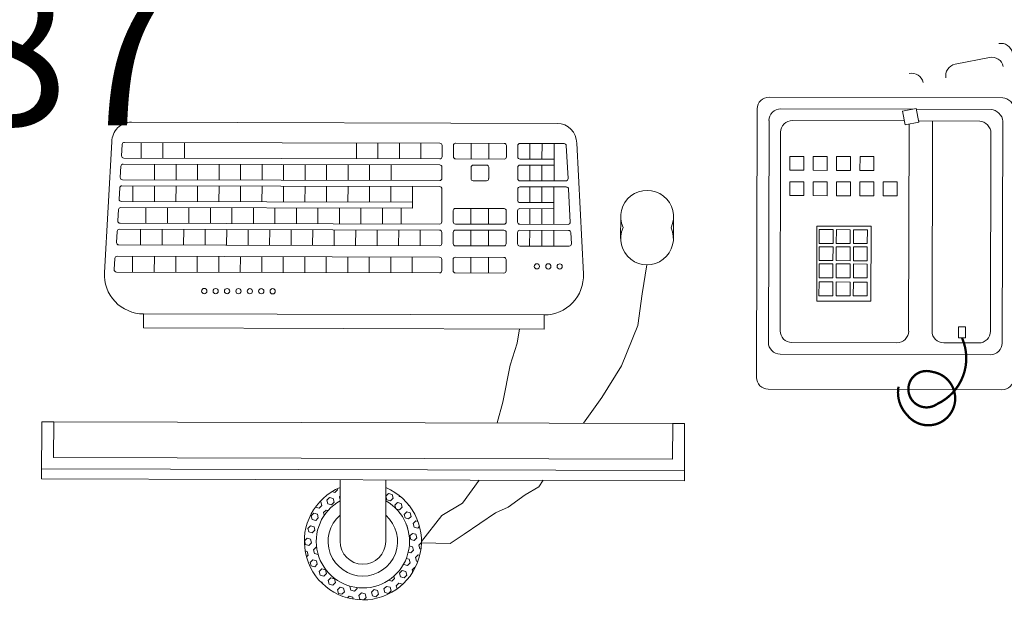
# Model space of a CAD drawing. Units: inches. Extents: x -466983 to 1020, y 324 to 318697.
# Tile 37 of 97: x 848 to 888, y 757 to 781. Entities that reach past the tile are written whole.
import ezdxf

# ---------------------------------------------------------------- set-up
doc = ezdxf.new("R2010")
doc.units = ezdxf.units.IN
doc.header["$MEASUREMENT"] = 0
for name, color, linetype, lineweight in [('A-ANNO-DIMS', 2, 'Continuous', 18), ('A-FLOR-PATT', 252, 'Continuous', 13), ('A-FURN', 8, 'Continuous', 18), ('CBV_01', 7, 'Continuous', 0)]:
    doc.layers.add(name, color=color, linetype=linetype, lineweight=lineweight)
doc.styles.get("Standard").update_dxf_attribs({"font": 'arial.ttf'})
doc.dimstyles.get("Standard").update_dxf_attribs({"dimtxt": 6, "dimasz": 4, "dimexe": 3, "dimexo": 3, "dimgap": 0.09, "dimtad": 0, "dimtih": 1, "dimtoh": 1, "dimdec": 1, "dimzin": 0, "dimdsep": 46, "dimlunit": 3, "dimtxsty": 'Standard', "dimcen": 0.09, "dimadec": 0, "dimazin": 0, "dimtfac": 1, "dimtdec": 1, "dimtofl": 0, "dimtmove": 0, "dimatfit": 3, "dimfxl": 1, "dimtolj": 1, "dimtzin": 0, "dimarcsym": 0})

# ---------------------------------------------------------------- blocks, each defined once
blk = doc.blocks.new('Offce Table')
at = {"layer": 'CBV_01'}
h = blk.add_hatch(dxfattribs=at)
h.set_pattern_fill('HEX', color=256, scale=1.206041, angle=-45.1538, style=0)
h.set_pattern_definition([(44.846232, (2370.5468, 299.66597), (0.18414034, -0.18513138), [0.1507551, -0.30151019]), (284.846232, (2370.5468, 299.66597), (-0.25239865, -0.06690453), [0.1507551, -0.30151019]), (344.846232, (2370.6537, 299.77229), (-0.06825831, -0.25203591), [0.1507551, -0.30151019])])
h.paths.add_polyline_path([(2601.472, 956.599), (2601.473, 957.136, -4.924372), (2599.622, 957.141), (2599.621, 956.604, 3.823416)])
for p, q in [((2625.938, 974.583, -0.016), (2624.545, 974.304, -0.016)), ((2626.476, 972.945, -0.016), (2617.003, 972.971, -0.016)), ((2616.528, 972.498, -0.016), (2616.499, 961.604, -0.016)), ((2622.832, 972.481, -0.016), (2617.475, 972.496, -0.016)), ((2626.001, 972.473, -0.016), (2622.97, 972.481, -0.016)), ((2591.166, 971.955, -0.016), (2608.412, 971.908, -0.016)), ((2617.001, 972.023, -0.016), (2616.976, 963.024, -0.016)), ((2622.49, 972.008, -0.016), (2617.948, 972.021, -0.016)), ((2622.661, 963.482, -0.016), (2622.684, 971.877, -0.016)), ((2625.552, 972, -0.016), (2623.065, 972.007, -0.016)), ((2623.609, 963.48, -0.016), (2623.632, 972.005, -0.016)), ((2626.449, 962.998, -0.016), (2626.473, 971.998, -0.016)), ((2617.473, 971.548, -0.016), (2617.451, 963.496, -0.016)), ((2625.977, 963.473, -0.016), (2625.998, 971.525, -0.016)), ((2590.067, 965.862, -0.016), (2590.368, 971.161, -0.016)), ((2590.761, 970.595, -0.016), (2590.787, 971.051, -0.016)), ((2590.877, 971.137, -0.016), (2603.66, 971.102, -0.016)), ((2591.557, 971.135, -0.016), (2591.555, 970.498, -0.016)), ((2592.439, 971.132, -0.016), (2592.437, 970.496, -0.016)), ((2593.31, 971.13, -0.016), (2593.309, 970.493, -0.016)), ((2600.28, 971.111, -0.016), (2600.278, 970.474, -0.016)), ((2601.151, 971.109, -0.016), (2601.15, 970.472, -0.016)), ((2602.023, 971.107, -0.016), (2602.021, 970.47, -0.016)), ((2602.894, 971.104, -0.016), (2602.892, 970.467, -0.016)), ((2603.75, 971.012, -0.016), (2603.749, 970.555, -0.016)), ((2604.211, 971.011, -0.016), (2604.21, 970.554, -0.016)), ((2604.302, 971.1, -0.016), (2606.269, 971.095, -0.016)), ((2604.928, 971.099, -0.016), (2604.926, 970.462, -0.016)), ((2605.643, 971.097, -0.016), (2605.642, 970.46, -0.016)), ((2606.359, 971.005, -0.016), (2606.358, 970.548, -0.016)), ((2606.821, 971.004, -0.016), (2606.82, 970.547, -0.016)), ((2606.911, 971.093, -0.016), (2608.697, 971.089, -0.016)), ((2607.311, 971.092, -0.016), (2607.31, 970.456, -0.016)), ((2607.802, 971.091, -0.016), (2607.8, 970.454, -0.016)), ((2608.292, 971.09, -0.016), (2608.288, 969.572, -0.016)), ((2608.855, 969.666, -0.016), (2608.787, 971.003, -0.016)), ((2609.478, 965.81, -0.016), (2609.206, 971.11, -0.016)), ((2590.851, 970.5, -0.016), (2603.658, 970.465, -0.016)), ((2590.711, 969.714, -0.016), (2590.737, 970.171, -0.016)), ((2590.827, 970.256, -0.016), (2603.657, 970.221, -0.016)), ((2592.1, 970.252, -0.016), (2592.098, 969.616, -0.016)), ((2592.971, 970.25, -0.016), (2592.97, 969.613, -0.016)), ((2593.842, 970.248, -0.016), (2593.841, 969.611, -0.016)), ((2594.714, 970.245, -0.016), (2594.712, 969.609, -0.016)), ((2595.585, 970.243, -0.016), (2595.583, 969.606, -0.016)), ((2596.456, 970.241, -0.016), (2596.454, 969.604, -0.016)), ((2597.327, 970.238, -0.016), (2597.326, 969.602, -0.016)), ((2598.199, 970.236, -0.016), (2598.197, 969.599, -0.016)), ((2599.07, 970.234, -0.016), (2599.068, 969.597, -0.016)), ((2599.941, 970.231, -0.016), (2599.939, 969.595, -0.016)), ((2600.812, 970.229, -0.016), (2600.811, 969.592, -0.016)), ((2601.683, 970.227, -0.016), (2601.682, 969.59, -0.016)), ((2603.747, 970.131, -0.016), (2603.746, 969.675, -0.016)), ((2604.3, 970.464, -0.016), (2606.267, 970.458, -0.016)), ((2604.925, 970.128, -0.016), (2604.924, 969.671, -0.016)), ((2605.015, 970.218, -0.016), (2605.551, 970.216, -0.016)), ((2605.641, 970.126, -0.016), (2605.64, 969.669, -0.016)), ((2606.818, 970.123, -0.016), (2606.817, 969.666, -0.016)), ((2606.909, 970.213, -0.016), (2608.289, 970.209, -0.016)), ((2606.91, 970.457, -0.016), (2608.29, 970.453, -0.016)), ((2607.309, 970.212, -0.016), (2607.307, 969.575, -0.016)), ((2607.799, 970.21, -0.016), (2607.798, 969.573, -0.016)), ((2590.777, 969.375, -0.016), (2603.655, 969.34, -0.016)), ((2590.801, 969.619, -0.016), (2603.656, 969.585, -0.016)), ((2591.215, 969.374, -0.016), (2591.214, 968.737, -0.016)), ((2592.098, 969.371, -0.016), (2592.096, 968.735, -0.016)), ((2592.969, 969.369, -0.016), (2592.967, 968.732, -0.016)), ((2593.84, 969.367, -0.016), (2593.838, 968.73, -0.016)), ((2594.711, 969.364, -0.016), (2594.71, 968.728, -0.016)), ((2595.583, 969.362, -0.016), (2595.581, 968.725, -0.016)), ((2596.454, 969.36, -0.016), (2596.452, 968.723, -0.016)), ((2597.325, 969.357, -0.016), (2597.323, 968.721, -0.016)), ((2598.196, 969.355, -0.016), (2598.195, 968.718, -0.016)), ((2599.067, 969.353, -0.016), (2599.066, 968.716, -0.016)), ((2599.939, 969.35, -0.016), (2599.937, 968.714, -0.016)), ((2600.81, 969.348, -0.016), (2600.808, 968.711, -0.016)), ((2601.681, 969.346, -0.016), (2601.679, 968.709, -0.016)), ((2602.552, 969.343, -0.016), (2602.55, 968.463, -0.016)), ((2605.014, 969.581, -0.016), (2605.549, 969.579, -0.016)), ((2606.907, 969.576, -0.016), (2608.765, 969.571, -0.016)), ((2606.907, 969.332, -0.016), (2608.787, 969.327, -0.016)), ((2607.307, 969.331, -0.016), (2607.305, 968.694, -0.016)), ((2607.797, 969.329, -0.016), (2607.795, 968.693, -0.016)), ((2608.287, 969.328, -0.016), (2608.283, 967.81, -0.016)), ((2590.661, 968.834, -0.016), (2590.687, 969.29, -0.016)), ((2603.745, 969.25, -0.016), (2603.741, 967.913, -0.016)), ((2606.816, 969.242, -0.016), (2606.815, 968.785, -0.016)), ((2608.946, 967.904, -0.016), (2608.877, 969.241, -0.016)), ((2590.727, 968.494, -0.016), (2602.55, 968.463, -0.016)), ((2590.751, 968.738, -0.016), (2602.551, 968.707, -0.016)), ((2606.905, 968.695, -0.016), (2608.285, 968.691, -0.016)), ((2590.611, 967.953, -0.016), (2590.637, 968.409, -0.016)), ((2591.751, 968.491, -0.016), (2591.75, 967.855, -0.016)), ((2592.623, 968.489, -0.016), (2592.621, 967.852, -0.016)), ((2593.494, 968.487, -0.016), (2593.492, 967.85, -0.016)), ((2594.365, 968.484, -0.016), (2594.363, 967.848, -0.016)), ((2595.236, 968.482, -0.016), (2595.235, 967.845, -0.016)), ((2596.108, 968.48, -0.016), (2596.106, 967.843, -0.016)), ((2596.979, 968.477, -0.016), (2596.977, 967.841, -0.016)), ((2597.85, 968.475, -0.016), (2597.848, 967.838, -0.016)), ((2598.721, 968.473, -0.016), (2598.719, 967.836, -0.016)), ((2599.592, 968.47, -0.016), (2599.591, 967.834, -0.016)), ((2600.464, 968.468, -0.016), (2600.462, 967.831, -0.016)), ((2601.335, 968.466, -0.016), (2601.333, 967.829, -0.016)), ((2602.092, 968.464, -0.016), (2602.091, 967.827, -0.016)), ((2604.204, 968.368, -0.016), (2604.203, 967.911, -0.016)), ((2604.295, 968.458, -0.016), (2606.262, 968.453, -0.016)), ((2604.92, 968.456, -0.016), (2604.919, 967.819, -0.016)), ((2605.636, 968.454, -0.016), (2605.635, 967.817, -0.016)), ((2606.352, 968.362, -0.016), (2606.351, 967.906, -0.016)), ((2606.814, 968.361, -0.016), (2606.813, 967.904, -0.016)), ((2606.904, 968.451, -0.016), (2608.285, 968.447, -0.016)), ((2607.304, 968.45, -0.016), (2607.303, 967.813, -0.016)), ((2607.794, 968.448, -0.016), (2607.793, 967.812, -0.016)), ((2610.991, 968.125, -0.016), (2610.989, 967.24, -0.016)), ((2613.126, 967.234, -0.016), (2613.129, 968.12, -0.016)), ((2590.701, 967.858, -0.016), (2603.651, 967.823, -0.016)), ((2604.293, 967.821, -0.016), (2606.26, 967.816, -0.016)), ((2606.902, 967.814, -0.016), (2608.855, 967.809, -0.016)), ((2618.946, 967.738, -0.016), (2618.938, 964.699, -0.016)), ((2621.142, 967.732, -0.016), (2618.946, 967.738, -0.016)), ((2621.134, 964.693, -0.016), (2621.142, 967.732, -0.016)), ((2590.561, 967.072, -0.016), (2590.587, 967.528, -0.016)), ((2590.677, 967.613, -0.016), (2603.65, 967.579, -0.016)), ((2591.526, 967.611, -0.016), (2591.525, 966.974, -0.016)), ((2592.409, 967.609, -0.016), (2592.407, 966.972, -0.016)), ((2593.28, 967.606, -0.016), (2593.278, 966.97, -0.016)), ((2594.151, 967.604, -0.016), (2594.149, 966.967, -0.016)), ((2595.022, 967.602, -0.016), (2595.021, 966.965, -0.016)), ((2595.893, 967.599, -0.016), (2595.892, 966.963, -0.016)), ((2596.765, 967.597, -0.016), (2596.763, 966.96, -0.016)), ((2597.636, 967.595, -0.016), (2597.634, 966.958, -0.016)), ((2598.507, 967.592, -0.016), (2598.505, 966.956, -0.016)), ((2599.378, 967.59, -0.016), (2599.377, 966.953, -0.016)), ((2600.25, 967.588, -0.016), (2600.248, 966.951, -0.016)), ((2601.121, 967.585, -0.016), (2601.119, 966.949, -0.016)), ((2601.992, 967.583, -0.016), (2601.99, 966.946, -0.016)), ((2602.863, 967.581, -0.016), (2602.862, 966.944, -0.016)), ((2603.74, 967.488, -0.016), (2603.739, 967.032, -0.016)), ((2604.202, 967.487, -0.016), (2604.201, 967.031, -0.016)), ((2604.292, 967.577, -0.016), (2606.26, 967.572, -0.016)), ((2604.918, 967.575, -0.016), (2604.916, 966.938, -0.016)), ((2605.634, 967.573, -0.016), (2605.632, 966.937, -0.016)), ((2606.35, 967.481, -0.016), (2606.348, 967.025, -0.016)), ((2606.811, 967.48, -0.016), (2606.81, 967.024, -0.016)), ((2606.902, 967.57, -0.016), (2608.878, 967.565, -0.016)), ((2607.302, 967.569, -0.016), (2607.3, 966.932, -0.016)), ((2607.792, 967.568, -0.016), (2607.79, 966.931, -0.016)), ((2608.282, 967.566, -0.016), (2608.281, 966.929, -0.016)), ((2608.991, 967.023, -0.016), (2608.968, 967.479, -0.016)), ((2590.651, 966.977, -0.016), (2603.649, 966.942, -0.016)), ((2604.291, 966.94, -0.016), (2606.258, 966.935, -0.016)), ((2606.9, 966.933, -0.016), (2608.901, 966.928, -0.016)), ((2590.579, 966.515, -0.016), (2603.647, 966.48, -0.016)), ((2591.208, 966.514, -0.016), (2591.206, 965.877, -0.016)), ((2592.09, 966.511, -0.016), (2592.088, 965.874, -0.016)), ((2592.961, 966.509, -0.016), (2592.959, 965.872, -0.016)), ((2593.832, 966.507, -0.016), (2593.831, 965.87, -0.016)), ((2594.704, 966.504, -0.016), (2594.702, 965.867, -0.016)), ((2595.575, 966.502, -0.016), (2595.573, 965.865, -0.016)), ((2596.446, 966.5, -0.016), (2596.444, 965.863, -0.016)), ((2590.463, 965.974, -0.016), (2590.489, 966.43, -0.016)), ((2597.317, 966.497, -0.016), (2597.316, 965.86, -0.016)), ((2598.189, 966.495, -0.016), (2598.187, 965.858, -0.016)), ((2599.06, 966.493, -0.016), (2599.058, 965.856, -0.016)), ((2599.931, 966.49, -0.016), (2599.929, 965.853, -0.016)), ((2600.802, 966.488, -0.016), (2600.8, 965.851, -0.016)), ((2601.673, 966.485, -0.016), (2601.672, 965.849, -0.016)), ((2602.545, 966.483, -0.016), (2602.543, 965.846, -0.016)), ((2603.737, 966.39, -0.016), (2603.736, 965.933, -0.016)), ((2604.199, 966.389, -0.016), (2604.198, 965.932, -0.016)), ((2604.289, 966.478, -0.016), (2606.257, 966.473, -0.016)), ((2604.915, 966.477, -0.016), (2604.913, 965.84, -0.016)), ((2605.631, 966.475, -0.016), (2605.629, 965.838, -0.016)), ((2606.347, 966.383, -0.016), (2606.346, 965.926, -0.016)), ((2590.553, 965.879, -0.016), (2603.646, 965.843, -0.016)), ((2604.288, 965.842, -0.016), (2606.255, 965.836, -0.016)), ((2618.938, 964.699, -0.016), (2621.134, 964.693, -0.016)), ((2591.651, 963.61, -0.016), (2591.652, 964.18, -0.016)), ((2591.652, 964.18, -0.016), (2607.884, 964.136, -0.016)), ((2607.883, 963.567, -0.016), (2607.884, 964.136, -0.016)), ((2591.651, 963.61, -0.016), (2607.883, 963.567, -0.016)), ((2617.924, 963.021, -0.016), (2622.186, 963.01, -0.016)), ((2624.081, 963.005, -0.016), (2625.502, 963.001, -0.016)), ((2617.449, 962.549, -0.016), (2625.974, 962.526, -0.016)), ((2616.971, 961.129, -0.016), (2626.444, 961.104, -0.016)), ((2587.523, 957.485, -0.016), (2587.529, 959.809, -0.016)), ((2588.012, 959.808, -0.016), (2587.529, 959.809, -0.016)), ((2588.008, 958.361, -0.016), (2588.012, 959.808, -0.016)), ((2613.097, 959.741, -0.016), (2588.012, 959.808, -0.016)), ((2613.093, 958.293, -0.016), (2613.097, 959.741, -0.016)), ((2613.097, 959.741, -0.016), (2613.58, 959.739, -0.016)), ((2613.574, 957.415, -0.016), (2613.58, 959.739, -0.016)), ((2613.093, 958.293, -0.016), (2588.008, 958.361, -0.016)), ((2613.575, 957.83, -0.016), (2587.524, 957.9, -0.016)), ((2613.574, 957.415, -0.016), (2587.523, 957.485, -0.016)), ((2599.623, 957.453, -0.016), (2599.616, 954.956, -0.016)), ((2601.467, 954.951, -0.016), (2601.474, 957.448, -0.016))]:
    blk.add_line(p, q, dxfattribs=at)
at = {"layer": 'CBV_01', "elevation": -0.016}
for points in [[(2622.965, 972.508), (2622.413, 972.397), (2622.523, 971.845), (2623.075, 971.955)], [(2618.41, 970.567), (2617.848, 970.568), (2617.846, 970.005), (2618.409, 970.004)], [(2619.358, 970.564), (2618.795, 970.566), (2618.794, 970.003), (2619.356, 970.001)], [(2620.305, 970.562), (2619.742, 970.563), (2619.741, 970), (2620.304, 969.999)], [(2621.252, 970.559), (2620.69, 970.561), (2620.688, 969.998), (2621.251, 969.996)], [(2618.408, 969.54), (2617.845, 969.541), (2617.843, 968.978), (2618.406, 968.977)], [(2619.355, 969.537), (2618.792, 969.539), (2618.791, 968.976), (2619.353, 968.974)], [(2620.302, 969.535), (2619.74, 969.536), (2619.738, 968.973), (2620.301, 968.972)], [(2621.25, 969.532), (2620.687, 969.534), (2620.685, 968.971), (2621.248, 968.969)], [(2622.197, 969.53), (2621.634, 969.531), (2621.633, 968.968), (2622.195, 968.967)], [(2619.597, 967.597), (2619.034, 967.599), (2619.032, 967.036), (2619.595, 967.034)], [(2620.292, 967.595), (2619.73, 967.597), (2619.728, 967.034), (2620.291, 967.032)], [(2620.988, 967.594), (2620.425, 967.595), (2620.424, 967.032), (2620.986, 967.031)], [(2619.595, 966.902), (2619.032, 966.904), (2619.031, 966.341), (2619.593, 966.339)], [(2620.29, 966.9), (2619.728, 966.902), (2619.726, 966.339), (2620.289, 966.337)], [(2620.986, 966.898), (2620.423, 966.9), (2620.422, 966.337), (2620.985, 966.335)], [(2619.593, 966.207), (2619.03, 966.208), (2619.029, 965.645), (2619.591, 965.644)], [(2620.289, 966.205), (2619.726, 966.207), (2619.724, 965.643), (2620.287, 965.642)], [(2620.984, 966.203), (2620.422, 966.205), (2620.42, 965.642), (2620.983, 965.64)], [(2619.591, 965.475), (2619.028, 965.477), (2619.027, 964.914), (2619.589, 964.912)], [(2620.287, 965.473), (2619.724, 965.475), (2619.722, 964.912), (2620.285, 964.91)], [(2620.982, 965.471), (2620.42, 965.473), (2620.418, 964.91), (2620.981, 964.908)], [(2624.959, 963.21), (2624.96, 963.66), (2624.678, 963.661), (2624.677, 963.211)]]:
    blk.add_lwpolyline(points, close=True, dxfattribs=at)
for points in [[(2612.055, 966.169), (2611.856, 964.989), (2611.679, 963.716), (2611.02, 962.076), (2610.22, 960.793), (2609.486, 959.75)], [(2606.891, 963.569), (2606.795, 962.987), (2606.508, 962.105), (2606.218, 960.599), (2605.987, 959.76)], [(2605.259, 957.437), (2604.573, 956.5), (2603.741, 956.009), (2602.914, 954.947)], [(2607.854, 957.43), (2607.669, 957.168), (2607.117, 956.845), (2606.434, 956.343), (2605.915, 956.117), (2604.644, 955.241), (2604.076, 954.87), (2602.914, 954.897)]]:
    blk.add_lwpolyline(points, dxfattribs=at)
at = {"layer": 'CBV_01', "const_width": 0.0942, "elevation": -0.016}
blk.add_lwpolyline([(2624.828, 963.196, -0.40574), (2623.816, 960.526, -1.618522), (2623.611, 961.83, -1.478802), (2622.602, 960.078, -0.24273), (2622.249, 961.227, -0.24273)], format="xyb", dxfattribs=at)
at = {"layer": 'CBV_01'}
for centre in [(2607.595, 966.107, -0.016), (2608.057, 966.106, -0.016), (2608.519, 966.105, -0.016), (2594.113, 965.106, -0.016), (2594.575, 965.104, -0.016), (2595.037, 965.103, -0.016), (2595.499, 965.102, -0.016), (2595.961, 965.101, -0.016), (2596.423, 965.099, -0.016), (2596.885, 965.098, -0.016)]:
    blk.add_circle(centre, 0.106, dxfattribs=at)
for centre, radius, start, end in [((2626.403, 974.675, -0.016), 0.474, 11.2965, 101.2965), ((2626.031, 974.118, -0.016), 0.474, 11.2965, 101.2965), ((2624.638, 973.84, -0.016), 0.474, 101.2965, 191.2965), ((2622.78, 973.469, -0.016), 0.474, 11.2965, 101.2965), ((2617.002, 972.497, -0.016), 0.474, 89.8453, 179.8453), ((2617.474, 972.022, -0.016), 0.474, 89.8453, 179.8453), ((2591.164, 971.159, -0.016), 0.796, 89.8462, 179.8462), ((2608.41, 971.112, -0.016), 0.796, 359.8462, 89.8462), ((2617.947, 971.547, -0.016), 0.474, 89.8453, 179.8453), ((2590.877, 971.046, -0.016), 0.0902, 89.8462, 176.7522), ((2603.66, 971.012, -0.016), 0.0902, 359.8462, 89.8462), ((2604.302, 971.01, -0.016), 0.0902, 89.8462, 179.8462), ((2606.269, 971.005, -0.016), 0.0902, 359.8462, 89.8462), ((2606.911, 971.003, -0.016), 0.0902, 89.8462, 179.8462), ((2608.696, 970.998, -0.016), 0.0902, 2.9403, 89.8462), ((2590.851, 970.59, -0.016), 0.0902, 176.7522, 269.8462), ((2603.658, 970.556, -0.016), 0.0902, 269.8462, 359.8462), ((2604.3, 970.554, -0.016), 0.0902, 179.8462, 269.8462), ((2606.268, 970.549, -0.016), 0.0902, 269.8462, 359.8462), ((2606.91, 970.547, -0.016), 0.0902, 179.8462, 269.8462), ((2590.827, 970.166, -0.016), 0.0902, 89.8462, 176.7522), ((2603.657, 970.131, -0.016), 0.0902, 359.8462, 89.8462), ((2605.015, 970.127, -0.016), 0.0902, 89.8462, 179.8462), ((2605.551, 970.126, -0.016), 0.0902, 359.8462, 89.8462), ((2606.909, 970.122, -0.016), 0.0902, 89.8462, 179.8462), ((2590.801, 969.709, -0.016), 0.0902, 176.7522, 269.8462), ((2590.777, 969.285, -0.016), 0.0902, 89.8462, 176.7522), ((2603.655, 969.25, -0.016), 0.0902, 359.8462, 89.8462), ((2603.656, 969.675, -0.016), 0.0902, 269.8462, 359.8462), ((2605.014, 969.671, -0.016), 0.0902, 179.8462, 269.8462), ((2605.549, 969.67, -0.016), 0.0902, 269.8462, 359.8462), ((2606.906, 969.241, -0.016), 0.0902, 89.8462, 179.8462), ((2606.907, 969.666, -0.016), 0.0902, 179.8462, 269.8462), ((2608.765, 969.661, -0.016), 0.0902, 269.8462, 2.9403), ((2608.787, 969.236, -0.016), 0.0902, 2.9403, 89.8462), ((2612.06, 968.122, -0.016), 1.069, 335.3844, 204.308), ((2590.727, 968.404, -0.016), 0.0902, 89.8462, 176.7522), ((2590.751, 968.828, -0.016), 0.0902, 176.7522, 269.8462), ((2606.905, 968.785, -0.016), 0.0902, 179.8462, 269.8462), ((2604.295, 968.368, -0.016), 0.0902, 89.8462, 179.8462), ((2606.262, 968.362, -0.016), 0.0902, 359.8462, 89.8462), ((2606.904, 968.361, -0.016), 0.0902, 89.8462, 179.8462), ((2590.701, 967.948, -0.016), 0.0902, 176.7522, 269.8462), ((2603.651, 967.913, -0.016), 0.0902, 269.8462, 359.8462), ((2604.293, 967.911, -0.016), 0.0902, 179.8462, 269.8462), ((2606.261, 967.906, -0.016), 0.0902, 269.8462, 359.8462), ((2606.903, 967.904, -0.016), 0.0902, 179.8462, 269.8462), ((2608.856, 967.899, -0.016), 0.0902, 269.8462, 2.9403), ((2590.677, 967.523, -0.016), 0.0902, 89.8462, 176.7522), ((2603.65, 967.488, -0.016), 0.0902, 359.8462, 89.8462), ((2604.292, 967.487, -0.016), 0.0902, 89.8462, 179.8462), ((2606.259, 967.481, -0.016), 0.0902, 359.8462, 89.8462), ((2606.902, 967.48, -0.016), 0.0902, 89.8462, 179.8462), ((2608.877, 967.474, -0.016), 0.0902, 2.9403, 89.8462), ((2612.058, 967.237, -0.016), 1.069, 155.3844, 24.308), ((2590.651, 967.067, -0.016), 0.0902, 176.7522, 269.8462), ((2603.649, 967.032, -0.016), 0.0902, 269.8462, 359.8462), ((2604.291, 967.03, -0.016), 0.0902, 179.8462, 269.8462), ((2606.258, 967.025, -0.016), 0.0902, 269.8462, 359.8462), ((2606.9, 967.023, -0.016), 0.0902, 179.8462, 269.8462), ((2608.901, 967.018, -0.016), 0.0902, 269.8462, 2.9403), ((2590.579, 966.425, -0.016), 0.0902, 89.8462, 176.7522), ((2603.647, 966.39, -0.016), 0.0902, 359.8462, 89.8462), ((2604.289, 966.388, -0.016), 0.0902, 89.8462, 179.8462), ((2606.257, 966.383, -0.016), 0.0902, 359.8462, 89.8462), ((2591.657, 965.772, -0.016), 1.592, 176.7522, 269.8462), ((2590.553, 965.969, -0.016), 0.0902, 176.7522, 269.8462), ((2603.646, 965.934, -0.016), 0.0902, 269.8462, 359.8462), ((2604.288, 965.932, -0.016), 0.0902, 179.8462, 269.8462), ((2606.255, 965.927, -0.016), 0.0902, 269.8462, 359.8462), ((2607.888, 965.728, -0.016), 1.592, 269.8462, 2.9403), ((2617.925, 963.495, -0.016), 0.474, 179.8453, 269.8453), ((2622.188, 963.484, -0.016), 0.474, 269.8453, 359.8453), ((2624.082, 963.478, -0.016), 0.474, 179.8453, 269.8453), ((2625.503, 963.475, -0.016), 0.474, 269.8453, 359.8453), ((2617.45, 963.023, -0.016), 0.474, 179.8453, 269.8453), ((2625.975, 963, -0.016), 0.474, 269.8453, 359.8453), ((2616.972, 961.603, -0.016), 0.474, 179.8453, 269.8453), ((2626.445, 961.578, -0.016), 0.474, 269.8453, 359.8453), ((2600.542, 954.954, -0.016), 2.373, 112.8043, 66.8881), ((2600.542, 954.954, -0.016), 1.89, 119.1606, 60.5319), ((2600.542, 954.954, -0.016), 1.408, 130.9449, 48.7475), ((2600.542, 954.954, -0.016), 0.926, 179.8462, 359.8462)]:
    blk.add_arc(centre, radius, start, end, dxfattribs=at)
for points in [[(2626.948, 972.47, -0.016), (2626.949, 972.693, -0.016), (2626.699, 972.944, -0.016), (2626.476, 972.945, -0.016)], [(2626.473, 971.998, -0.016), (2626.474, 972.221, -0.016), (2626.224, 972.472, -0.016), (2626.001, 972.473, -0.016)], [(2625.998, 971.525, -0.016), (2625.999, 971.743, -0.016), (2625.769, 972, -0.016), (2625.552, 972, -0.016)]]:
    blk.add_open_spline(points, degree=3, dxfattribs=at)
blk = doc.blocks.new('Office Desk With Chairs')
blk.add_blockref('Offce Table', (-526.404, 94.584))
blk = doc.blocks.new('*D91')
at = {"layer": 'A-ANNO-DIMS', "color": 0, "lineweight": -2, "transparency": 16777216}
for p, q in [((938.253, 802.547), (920.07, 802.547)), ((923.07, 798.547), (923.07, 745.132)), ((923.07, 685.328), (923.07, 738.743)), ((938.253, 681.328), (920.07, 681.328))]:
    blk.add_line(p, q, dxfattribs=at)
at = {"layer": 'A-ANNO-DIMS', "color": 0, "transparency": 16777216}
for points in [[(922.404, 798.547), (923.737, 798.547), (923.07, 802.547)], [(922.404, 685.328), (923.737, 685.328), (923.07, 681.328)]]:
    blk.add_solid(points, dxfattribs=at)
at = {"layer": 'Defpoints', "color": 0, "transparency": 16777216}
for p in [(941.253, 802.547), (923.07, 681.328), (941.253, 681.328)]:
    blk.add_point(p, dxfattribs=at)
at = {"layer": 'A-ANNO-DIMS', "color": 0, "transparency": 16777216, "insert": (923.07, 741.937), "char_height": 6, "attachment_point": 5}
blk.add_mtext('\\A1;4-SEATER SOFA 121', dxfattribs=at)
blk = doc.blocks.new('*D99')
at = {"layer": 'A-ANNO-DIMS', "color": 0, "lineweight": -2, "transparency": 16777216}
for p, q in [((833.84, 822.679), (820.85, 822.679)), ((823.85, 818.679), (823.85, 782.572)), ((823.85, 740.077), (823.85, 776.184)), ((833.84, 736.077), (820.85, 736.077))]:
    blk.add_line(p, q, dxfattribs=at)
at = {"layer": 'A-ANNO-DIMS', "color": 0, "transparency": 16777216}
for points in [[(823.183, 818.679), (824.517, 818.679), (823.85, 822.679)], [(823.183, 740.077), (824.517, 740.077), (823.85, 736.077)]]:
    blk.add_solid(points, dxfattribs=at)
at = {"layer": 'Defpoints', "color": 0, "transparency": 16777216}
for p in [(823.85, 822.679), (836.84, 822.679), (836.84, 736.077)]:
    blk.add_point(p, dxfattribs=at)
at = {"layer": 'A-ANNO-DIMS', "color": 0, "transparency": 16777216, "insert": (823.85, 779.378), "char_height": 6, "attachment_point": 5}
blk.add_mtext('\\A1;OFFICE DESK 87', dxfattribs=at)

msp = doc.modelspace()

# ---------------------------------------------------------------- hatches: boundary and pattern name
at = {"layer": 'A-FLOR-PATT', "transparency": 33554572}
h = msp.add_hatch(dxfattribs=at)
h.set_pattern_fill('ANSI37', color=256, scale=30)
h.set_pattern_definition([(45, (-1212.4137, -290.035), (-2.6516504, 2.6516504), []), (135, (-1212.4137, -290.035), (-2.6516504, -2.6516504), [])])
h.paths.add_polyline_path([(901.806, 1075.938), (900.614, 1075.938), (900.614, 1065.386), (899.391, 1065.386), (898.091, 1065.386), (892.836, 1058.71, -0.258377), (892.188, 1058.351), (879.985, 1058.351, -0.20177), (879.438, 1058.581), (874.081, 1065.386), (872.781, 1065.386), (871.558, 1065.386), (871.558, 1075.938), (813.806, 1075.938), (813.806, 1044.792), (832.395, 1044.792, -0.394795), (848.66, 1028.536), (848.66, 1009.938), (901.806, 1009.938), (901.806, 1015.938), (901.306, 1015.938), (871.306, 1015.938), (871.306, 1017.25), (871.334, 1017.25, -0.401453), (901.306, 1045.938), (901.806, 1045.938)])
edge = h.paths.add_edge_path(flags=16)
edge.add_line((847.773, 1068.949), (847.773, 1073.709))
edge.add_arc((849.227, 1073.709), 1.454, 90, 180, ccw=False)
edge.add_line((849.227, 1075.163), (864.492, 1075.163))
edge.add_arc((864.492, 1073.709), 1.454, 0, 90, ccw=False)
edge.add_line((865.946, 1073.709), (865.946, 1069.004))
edge.add_arc((832.645, 1068.976), 33.301, -20.6123, 0.0472, ccw=False)
edge.add_ellipse((856.859, 1058.48), major_axis=(0, 10.213), ratio=0.685919, start_angle=100.0088, end_angle=259.9912, ccw=False)
edge.add_arc((881.074, 1068.976), 33.301, 180.0472, 200.6123, ccw=False)
h.paths.add_polyline_path([(853.146, 1066.482), (853.146, 1066.453), (853.146, 1066.453, 0.433107), (852.917, 1066.685), (852.917, 1066.453), (853.146, 1066.453), (853.146, 1066.482), (853.088, 1066.612, 0.697939), (852.7, 1066.453), (852.7, 1066.453), (852.7, 1066.482), (852.917, 1067.001), (852.917, 1066.685, -0.396254)], flags=0)
h.paths.add_polyline_path([(861.019, 1066.482), (861.019, 1066.453), (861.019, 1066.453, 0.416404), (860.802, 1066.685), (860.802, 1066.453), (861.019, 1066.453), (861.019, 1066.482), (860.967, 1066.605, 0.713344), (860.573, 1066.453), (860.573, 1066.453), (860.573, 1066.482), (860.802, 1067.001), (860.802, 1066.685, -0.379973)], flags=0)
edge = h.paths.add_edge_path(flags=0)
edge.add_spline(control_points=[(861.13, 1065.785), (861.466, 1065.248), (861.613, 1065.016), (861.983, 1064.374), (862.192, 1063.944), (862.561, 1063.039), (862.721, 1062.563), (862.987, 1061.578), (863.092, 1061.069), (863.245, 1060.031), (863.293, 1059.503), (863.329, 1058.441), (863.318, 1057.908), (863.237, 1056.852), (863.166, 1056.329), (862.97, 1055.308), (862.843, 1054.81), (862.537, 1053.852), (862.357, 1053.393), (861.951, 1052.525), (861.725, 1052.117), (861.233, 1051.362), (860.967, 1051.016), (860.405, 1050.395), (860.108, 1050.12), (859.494, 1049.646), (859.176, 1049.448), (858.528, 1049.13), (858.197, 1049.011), (857.531, 1048.852), (857.196, 1048.812), (856.525, 1048.812), (856.189, 1048.852), (855.524, 1049.01), (855.193, 1049.129), (854.545, 1049.447), (854.227, 1049.645), (853.612, 1050.118), (853.316, 1050.393), (852.753, 1051.014), (852.487, 1051.36), (851.995, 1052.114), (851.769, 1052.523), (851.363, 1053.39), (851.183, 1053.85), (850.877, 1054.807), (850.75, 1055.305), (850.553, 1056.326), (850.483, 1056.849), (850.401, 1057.905), (850.39, 1058.438), (850.426, 1059.5), (850.473, 1060.028), (850.626, 1061.066), (850.732, 1061.575), (850.997, 1062.561), (851.157, 1063.036), (851.525, 1063.942), (851.734, 1064.371), (852.106, 1065.016), (852.254, 1065.25), (852.608, 1065.733)], knot_values=[3.915332, 3.915332, 3.915332, 3.915332, 4.013468, 4.013468, 4.175532, 4.175532, 4.337596, 4.337596, 4.49966, 4.49966, 4.661724, 4.661724, 4.823788, 4.823788, 4.985852, 4.985852, 5.147916, 5.147916, 5.30998, 5.30998, 5.472044, 5.472044, 5.634109, 5.634109, 5.796173, 5.796173, 5.958237, 5.958237, 6.120301, 6.120301, 6.282365, 6.282365, 6.444429, 6.444429, 6.606493, 6.606493, 6.768557, 6.768557, 6.930621, 6.930621, 7.092685, 7.092685, 7.254749, 7.254749, 7.416813, 7.416813, 7.578878, 7.578878, 7.740942, 7.740942, 7.903006, 7.903006, 8.06507, 8.06507, 8.227134, 8.227134, 8.389198, 8.389198, 8.551262, 8.551262, 8.65037, 8.65037, 8.65037, 8.65037], degree=3, periodic=0)
edge.add_line((852.642, 1065.785), (861.13, 1065.785))
edge = h.paths.add_edge_path(flags=0)
edge.add_ellipse((856.85, 1057.743), major_axis=(0, 7.792), ratio=0.687861, start_angle=0, end_angle=360)
h.paths.add_polyline_path([(848.863, 1069.389), (848.863, 1073.96, -0.414214), (849.954, 1075.051), (863.765, 1075.051, -0.414214), (864.856, 1073.96), (864.856, 1069.389, -0.388936), (864.524, 1069.027, -0.043561), (849.195, 1069.027, -0.388936)], flags=0)
h.paths.add_polyline_path([(853.101, 1068.112, -1), (852.677, 1068.112, -1)], flags=0)
edge = h.paths.add_edge_path(flags=0)
edge.add_ellipse((856.859, 1057.338), major_axis=(0, 2.207), ratio=0.657164, start_angle=0, end_angle=360)
h.paths.add_polyline_path([(861.041, 1068.112, -1), (860.618, 1068.112, -1)], flags=0)
edge = h.paths.add_edge_path()
edge.add_line((573.954, 1057.341), (573.954, 1075.938))
edge.add_line((573.954, 1075.938), (558.731, 1075.938))
edge.add_line((558.731, 1075.938), (558.731, 1065.386))
edge.add_line((558.731, 1065.386), (557.507, 1065.386))
edge.add_line((557.507, 1065.386), (556.207, 1065.386))
edge.add_line((556.207, 1065.386), (550.952, 1058.71))
edge.add_arc((550.304, 1059.116), 0.765, 270, 327.9483, ccw=False)
edge.add_line((550.304, 1058.351), (538.101, 1058.351))
edge.add_arc((538.101, 1059.116), 0.765, 224.3704, 270, ccw=False)
edge.add_line((537.555, 1058.581), (532.198, 1065.386))
edge.add_line((532.198, 1065.386), (530.898, 1065.386))
edge.add_line((530.898, 1065.386), (529.674, 1065.386))
edge.add_line((529.674, 1065.386), (529.674, 1075.938))
edge.add_line((529.674, 1075.938), (520.806, 1075.938))
edge.add_line((520.806, 1075.938), (520.806, 1045.938))
edge.add_line((520.806, 1045.938), (521.306, 1045.938))
edge.add_arc((521.306, 1015.938), 30, 2.5075, 90, ccw=False)
edge.add_line((551.277, 1017.25), (551.306, 1017.25))
edge.add_line((551.306, 1017.25), (551.306, 1015.938))
edge.add_line((551.306, 1015.938), (520.806, 1015.938))
edge.add_line((520.806, 1015.938), (520.806, 1009.938))
edge.add_line((520.806, 1009.938), (559.191, 1010.402))
edge.add_arc((559.191, 1011.856), 1.454, 180, 270, ccw=False)
edge.add_line((557.737, 1011.856), (557.737, 1016.561))
edge.add_arc((591.039, 1016.589), 33.301, 159.3877, 180.0472, ccw=False)
edge.add_ellipse((566.824, 1027.085), major_axis=(0, 10.213), ratio=0.685919, start_angle=280.0088, end_angle=439.9912, ccw=False)
edge.add_arc((542.609, 1016.589), 33.301, 0.0472, 20.6123, ccw=False)
edge.add_line((575.91, 1016.616), (575.91, 1011.856))
edge.add_arc((574.456, 1011.856), 1.454, -90, 0, ccw=False)
edge.add_line((574.456, 1010.402), (608.806, 1009.938))
edge.add_line((608.806, 1009.938), (608.806, 1041.086))
edge.add_line((608.806, 1041.086), (590.218, 1041.086))
edge.add_arc((590.775, 1057.907), 16.831, 181.9277, 268.1032, ccw=False)
edge = h.paths.add_edge_path()
edge.add_ellipse((494.244, 583.62), major_axis=(0, 10.213), ratio=0.685919, start_angle=280.0088, end_angle=439.9912, ccw=False)
edge.add_arc((470.03, 573.124), 33.301, 0.0472, 20.6123, ccw=False)
edge.add_line((503.331, 573.152), (503.331, 568.392))
edge.add_arc((501.877, 568.392), 1.454, -90, 0, ccw=False)
edge.add_line((501.877, 566.938), (539.806, 566.938))
edge.add_line((539.806, 566.938), (539.806, 572.938))
edge.add_line((539.806, 572.938), (539.306, 572.938))
edge.add_line((539.306, 572.938), (509.306, 572.938))
edge.add_line((509.306, 572.938), (509.306, 574.25))
edge.add_line((509.306, 574.25), (509.334, 574.25))
edge.add_arc((539.306, 572.938), 30, 90, 177.4925, ccw=False)
edge.add_line((539.306, 602.938), (539.806, 602.938))
edge.add_line((539.806, 602.938), (539.806, 626.938))
edge.add_line((539.806, 626.938), (531.772, 626.938))
edge.add_line((531.772, 626.938), (531.772, 616.386))
edge.add_line((531.772, 616.386), (530.548, 616.386))
edge.add_line((530.548, 616.386), (529.249, 616.386))
edge.add_line((529.249, 616.386), (523.711, 609.351))
edge.add_line((523.711, 609.351), (510.777, 609.351))
edge.add_line((510.777, 609.351), (505.239, 616.386))
edge.add_line((505.239, 616.386), (503.939, 616.386))
edge.add_line((503.939, 616.386), (502.715, 616.386))
edge.add_line((502.715, 616.386), (502.715, 626.938))
edge.add_line((502.715, 626.938), (481.698, 626.938))
edge.add_line((481.698, 626.938), (481.698, 610.995))
edge.add_arc((467.27, 611.473), 14.436, 271.9277, 358.1032, ccw=False)
edge.add_line((467.756, 597.045), (451.806, 597.045))
edge.add_line((451.806, 597.045), (451.806, 584.404))
edge.add_line((451.806, 584.404), (451.806, 566.938))
edge.add_line((451.806, 566.938), (486.612, 566.938))
edge.add_arc((486.612, 568.392), 1.454, 180, 270, ccw=False)
edge.add_line((485.158, 568.392), (485.158, 573.097))
edge.add_arc((518.459, 573.124), 33.301, 159.3877, 180.0472, ccw=False)
h.paths.add_polyline_path([(836.261, 1020.733), (879.89, 1020.733), (879.89, 1039.39), (836.261, 1039.39)], flags=25)
h.paths.add_polyline_path([(549.985, 1036.749), (593.614, 1036.749), (593.614, 1055.407), (549.985, 1055.407)], flags=24)
h.paths.add_polyline_path([(475.123, 595.596), (518.752, 595.596), (518.752, 614.253), (475.123, 614.253)], flags=24)

# ---------------------------------------------------------------- block references
at = {"layer": 'A-FURN'}
msp.add_blockref('Office Desk With Chairs', (-1212.414, -290.035), dxfattribs=at)

# ---------------------------------------------------------------- dimensions: what is measured, and where the dimension line sits
at = {"layer": 'A-ANNO-DIMS'}
for base, p1, p2, angle, text, picture, middle in [((823.85, 822.679), (836.84, 736.077), (836.84, 822.679), 90, 'OFFICE DESK <>', '*D99', (823.85, 779.378)), ((923.07, 681.328), (941.253, 802.547), (941.253, 681.328), 270, '4-SEATER SOFA <>', '*D91', (923.07, 741.937))]:
    dim = msp.add_linear_dim(base=base, p1=p1, p2=p2, angle=angle, text=text, dimstyle='Standard', override={"dimdec": 0, "dimlfac": 1, "dimrnd": 0, "dimzin": 0, "dimdsep": 46, "dimlunit": 2}, dxfattribs=at)
    dim.commit()
    dim.dimension.update_dxf_attribs({"geometry": picture, "text_midpoint": middle})

doc.saveas('drawing.dxf')
